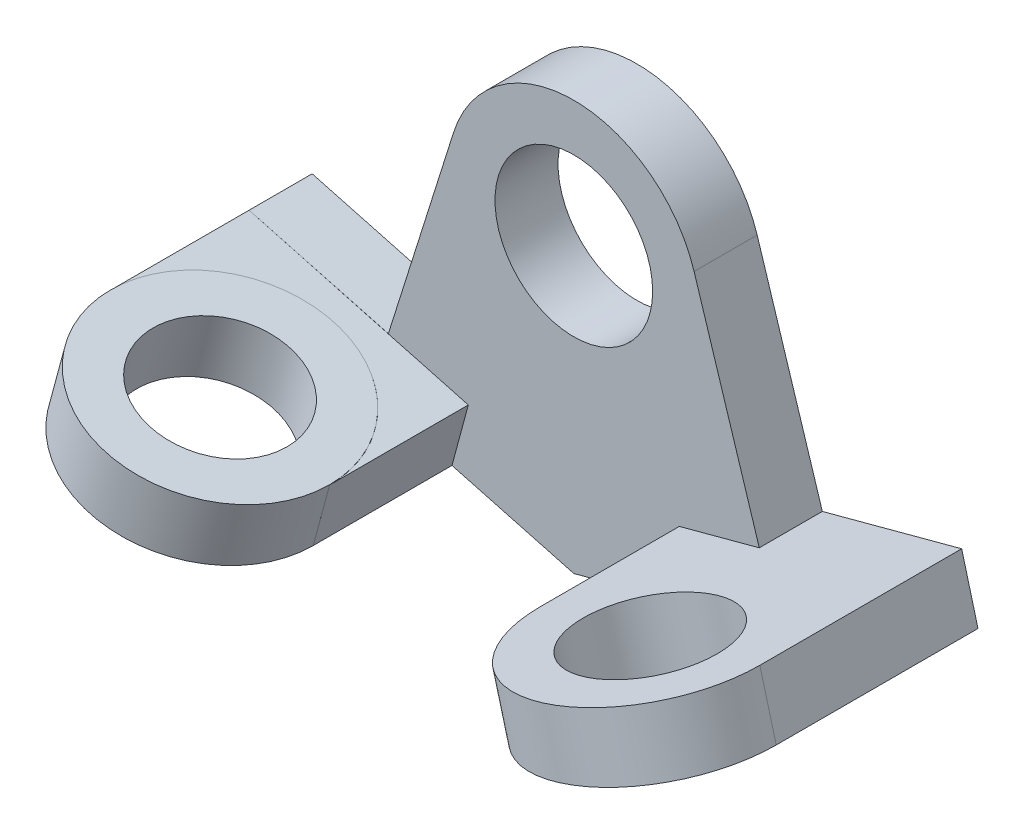
ISO-10303-21;
HEADER;
FILE_DESCRIPTION(('STEP AP214'),'2;1');
FILE_NAME('part.step','',(''),(''),'','','');
FILE_SCHEMA(('AUTOMOTIVE_DESIGN { 1 0 10303 214 1 1 1 1 }'));
ENDSEC;
DATA;
#1=APPLICATION_CONTEXT('core data for automotive mechanical design processes');
#2=APPLICATION_PROTOCOL_DEFINITION('international standard','automotive_design',2000,#1);
#3=PRODUCT_CONTEXT('',#1,'mechanical');
#4=PRODUCT('Part','Part','',(#3));
#5=PRODUCT_RELATED_PRODUCT_CATEGORY('part','',(#4));
#6=PRODUCT_DEFINITION_FORMATION('','',#4);
#7=PRODUCT_DEFINITION_CONTEXT('part definition',#1,'design');
#8=PRODUCT_DEFINITION('design','',#6,#7);
#9=PRODUCT_DEFINITION_SHAPE('','',#8);
#10=(LENGTH_UNIT() NAMED_UNIT(*) SI_UNIT(.MILLI.,.METRE.));
#11=(NAMED_UNIT(*) PLANE_ANGLE_UNIT() SI_UNIT($,.RADIAN.));
#12=(NAMED_UNIT(*) SI_UNIT($,.STERADIAN.) SOLID_ANGLE_UNIT());
#13=UNCERTAINTY_MEASURE_WITH_UNIT(LENGTH_MEASURE(1.E-05),#10,'distance_accuracy_value','');
#14=(GEOMETRIC_REPRESENTATION_CONTEXT(3) GLOBAL_UNCERTAINTY_ASSIGNED_CONTEXT((#13)) GLOBAL_UNIT_ASSIGNED_CONTEXT((#10,
#11,#12)) REPRESENTATION_CONTEXT('',''));
#15=CARTESIAN_POINT('',(0.,0.,0.));
#16=DIRECTION('',(0.,0.,1.));
#17=DIRECTION('',(1.,0.,0.));
#18=AXIS2_PLACEMENT_3D('',#15,#16,#17);
#19=CARTESIAN_POINT('',(0.,0.,10.));
#20=DIRECTION('',(0.,0.,1.));
#21=DIRECTION('',(1.,0.,0.));
#22=AXIS2_PLACEMENT_3D('',#19,#20,#21);
#23=PLANE('',#22);
#24=CARTESIAN_POINT('',(0.,45.,10.));
#25=DIRECTION('',(0.,0.,1.));
#26=DIRECTION('',(1.,0.,0.));
#27=AXIS2_PLACEMENT_3D('',#24,#25,#26);
#28=CIRCLE('',#27,12.5);
#29=CARTESIAN_POINT('',(12.5,45.,10.));
#30=VERTEX_POINT('',#29);
#31=EDGE_CURVE('E424',#30,#30,#28,.T.);
#32=ORIENTED_EDGE('',*,*,#31,.F.);
#33=EDGE_LOOP('',(#32));
#34=FACE_BOUND('',#33,.T.);
#35=DIRECTION('',(0.258819045102522,-0.965925826289068,0.));
#36=VECTOR('',#35,1.);
#37=CARTESIAN_POINT('',(16.7303260747562,14.8356391649411,10.));
#38=LINE('',#37,#36);
#39=CARTESIAN_POINT('',(16.7303260747562,14.8356391649411,10.));
#40=VERTEX_POINT('',#39);
#41=CARTESIAN_POINT('',(19.3185165257814,5.17638090205043,10.));
#42=VERTEX_POINT('',#41);
#43=EDGE_CURVE('E172',#40,#42,#38,.T.);
#44=ORIENTED_EDGE('',*,*,#43,.F.);
#45=DIRECTION('',(-0.965925826289068,-0.258819045102522,0.));
#46=VECTOR('',#45,1.);
#47=CARTESIAN_POINT('',(51.5036558211626,24.1531247886319,10.));
#48=LINE('',#47,#46);
#49=CARTESIAN_POINT('',(29.4101278592332,18.2331818132785,10.));
#50=VERTEX_POINT('',#49);
#51=EDGE_CURVE('E210',#50,#40,#48,.T.);
#52=ORIENTED_EDGE('',*,*,#51,.F.);
#53=DIRECTION('',(0.300705799504267,-0.953716950748229,0.));
#54=VECTOR('',#53,1.);
#55=CARTESIAN_POINT('',(31.9798088328629,10.0831949935828,10.));
#56=LINE('',#55,#54);
#57=CARTESIAN_POINT('',(19.0743390149646,51.0141159900853,10.));
#58=VERTEX_POINT('',#57);
#59=EDGE_CURVE('E284',#58,#50,#56,.T.);
#60=ORIENTED_EDGE('',*,*,#59,.F.);
#61=CARTESIAN_POINT('',(0.,45.,10.));
#62=DIRECTION('',(0.,0.,1.));
#63=DIRECTION('',(1.,0.,0.));
#64=AXIS2_PLACEMENT_3D('',#61,#62,#63);
#65=CIRCLE('',#64,20.);
#66=CARTESIAN_POINT('',(-19.0743390149646,51.0141159900853,10.));
#67=VERTEX_POINT('',#66);
#68=EDGE_CURVE('E337',#58,#67,#65,.T.);
#69=ORIENTED_EDGE('',*,*,#68,.T.);
#70=DIRECTION('',(-0.300705799504267,-0.953716950748229,0.));
#71=VECTOR('',#70,1.);
#72=CARTESIAN_POINT('',(-31.9798088328629,10.0831949935828,10.));
#73=LINE('',#72,#71);
#74=CARTESIAN_POINT('',(-29.4101278592332,18.2331818132785,10.));
#75=VERTEX_POINT('',#74);
#76=EDGE_CURVE('E271',#67,#75,#73,.T.);
#77=ORIENTED_EDGE('',*,*,#76,.T.);
#78=DIRECTION('',(-0.965925826289068,0.258819045102521,0.));
#79=VECTOR('',#78,1.);
#80=CARTESIAN_POINT('',(2.58819045102521,9.65925826289068,10.));
#81=LINE('',#80,#79);
#82=CARTESIAN_POINT('',(-51.4905816094325,24.1496215641571,10.));
#83=VERTEX_POINT('',#82);
#84=EDGE_CURVE('E320',#75,#83,#81,.T.);
#85=ORIENTED_EDGE('',*,*,#84,.T.);
#86=DIRECTION('',(-0.965573757302424,0.260129427802544,0.));
#87=VECTOR('',#86,1.);
#88=CARTESIAN_POINT('',(-51.4905816094325,24.1496215641571,10.));
#89=LINE('',#88,#87);
#90=CARTESIAN_POINT('',(-16.7299263465452,14.7849621632655,10.));
#91=VERTEX_POINT('',#90);
#92=EDGE_CURVE('E357',#91,#83,#89,.T.);
#93=ORIENTED_EDGE('',*,*,#92,.F.);
#94=DIRECTION('',(0.260129427802545,0.965573757302424,0.));
#95=VECTOR('',#94,1.);
#96=CARTESIAN_POINT('',(-16.7299263465452,14.7849621632655,10.));
#97=LINE('',#96,#95);
#98=CARTESIAN_POINT('',(-19.3181864512745,5.17760610474064,10.));
#99=VERTEX_POINT('',#98);
#100=EDGE_CURVE('E365',#99,#91,#97,.T.);
#101=ORIENTED_EDGE('',*,*,#100,.F.);
#102=DIRECTION('',(0.965582925438563,-0.260095394233551,0.));
#103=VECTOR('',#102,1.);
#104=CARTESIAN_POINT('',(-54.079171788662,14.5410403029666,10.));
#105=LINE('',#104,#103);
#106=CARTESIAN_POINT('',(-54.079171788662,14.5410403029666,10.));
#107=VERTEX_POINT('',#106);
#108=EDGE_CURVE('E346',#107,#99,#105,.T.);
#109=ORIENTED_EDGE('',*,*,#108,.F.);
#110=DIRECTION('',(-0.96557375730224,0.260129427803227,0.));
#111=VECTOR('',#110,1.);
#112=CARTESIAN_POINT('',(-0.00705915648429595,-0.0262028648872519,10.));
#113=LINE('',#112,#111);
#114=CARTESIAN_POINT('',(-32.4145115016567,8.70449426866302,10.));
#115=VERTEX_POINT('',#114);
#116=EDGE_CURVE('E312',#115,#107,#113,.T.);
#117=ORIENTED_EDGE('',*,*,#116,.F.);
#118=CARTESIAN_POINT('',(-32.420050633813,8.68692638590632,10.));
#119=VERTEX_POINT('',#118);
#120=EDGE_CURVE('E297',#115,#119,#73,.T.);
#121=ORIENTED_EDGE('',*,*,#120,.T.);
#122=DIRECTION('',(-0.965925826289068,0.258819045102521,0.));
#123=VECTOR('',#122,1.);
#124=CARTESIAN_POINT('',(0.,0.,10.));
#125=LINE('',#124,#123);
#126=CARTESIAN_POINT('',(0.,0.,10.));
#127=VERTEX_POINT('',#126);
#128=EDGE_CURVE('E295',#127,#119,#125,.T.);
#129=ORIENTED_EDGE('',*,*,#128,.F.);
#130=DIRECTION('',(0.965925826289068,0.258819045102521,0.));
#131=VECTOR('',#130,1.);
#132=CARTESIAN_POINT('',(0.,0.,10.));
#133=LINE('',#132,#131);
#134=EDGE_CURVE('E290',#127,#42,#133,.T.);
#135=ORIENTED_EDGE('',*,*,#134,.T.);
#136=EDGE_LOOP('',(#44,#52,#60,#69,#77,#85,#93,#101,#109,#117,#121,#129,#135));
#137=FACE_BOUND('',#136,.T.);
#138=ADVANCED_FACE('F41',(#34,#137),#23,.T.);
#139=CARTESIAN_POINT('',(31.9798088328629,10.0831949935828,10.));
#140=DIRECTION('',(0.953716950748229,0.300705799504267,0.));
#141=DIRECTION('',(-0.300705799504267,0.953716950748229,0.));
#142=AXIS2_PLACEMENT_3D('',#139,#140,#141);
#143=PLANE('',#142);
#144=ORIENTED_EDGE('',*,*,#59,.T.);
#145=DIRECTION('',(0.,0.,-1.));
#146=VECTOR('',#145,1.);
#147=CARTESIAN_POINT('',(29.4101278592332,18.2331818132785,10.));
#148=LINE('',#147,#146);
#149=CARTESIAN_POINT('',(29.4101278592332,18.2331818132785,0.));
#150=VERTEX_POINT('',#149);
#151=EDGE_CURVE('E315',#50,#150,#148,.T.);
#152=ORIENTED_EDGE('',*,*,#151,.T.);
#153=DIRECTION('',(0.300705799504267,-0.953716950748229,0.));
#154=VECTOR('',#153,1.);
#155=CARTESIAN_POINT('',(31.9798088328629,10.0831949935828,0.));
#156=LINE('',#155,#154);
#157=CARTESIAN_POINT('',(19.0743390149646,51.0141159900853,0.));
#158=VERTEX_POINT('',#157);
#159=EDGE_CURVE('E264',#158,#150,#156,.T.);
#160=ORIENTED_EDGE('',*,*,#159,.F.);
#161=DIRECTION('',(0.,0.,-1.));
#162=VECTOR('',#161,1.);
#163=CARTESIAN_POINT('',(19.0743390149646,51.0141159900853,10.));
#164=LINE('',#163,#162);
#165=EDGE_CURVE('E47',#58,#158,#164,.T.);
#166=ORIENTED_EDGE('',*,*,#165,.F.);
#167=EDGE_LOOP('',(#144,#152,#160,#166));
#168=FACE_BOUND('',#167,.T.);
#169=ADVANCED_FACE('F43',(#168),#143,.T.);
#170=CARTESIAN_POINT('',(-31.9798088328629,10.0831949935828,10.));
#171=DIRECTION('',(0.953716950748229,-0.300705799504267,0.));
#172=DIRECTION('',(0.300705799504267,0.953716950748229,0.));
#173=AXIS2_PLACEMENT_3D('',#170,#171,#172);
#174=PLANE('',#173);
#175=DIRECTION('',(0.,0.,1.));
#176=VECTOR('',#175,1.);
#177=CARTESIAN_POINT('',(-32.4145115016567,8.70449426866302,10.));
#178=LINE('',#177,#176);
#179=CARTESIAN_POINT('',(-32.4145115016567,8.70449426866302,0.));
#180=VERTEX_POINT('',#179);
#181=EDGE_CURVE('E299',#180,#115,#178,.T.);
#182=ORIENTED_EDGE('',*,*,#181,.F.);
#183=DIRECTION('',(-0.300705799504267,-0.953716950748229,0.));
#184=VECTOR('',#183,1.);
#185=CARTESIAN_POINT('',(-31.9798088328629,10.0831949935828,0.));
#186=LINE('',#185,#184);
#187=CARTESIAN_POINT('',(-32.420050633813,8.68692638590632,0.));
#188=VERTEX_POINT('',#187);
#189=EDGE_CURVE('E262',#180,#188,#186,.T.);
#190=ORIENTED_EDGE('',*,*,#189,.T.);
#191=DIRECTION('',(0.,0.,-1.));
#192=VECTOR('',#191,1.);
#193=CARTESIAN_POINT('',(-32.420050633813,8.68692638590632,10.));
#194=LINE('',#193,#192);
#195=EDGE_CURVE('E275',#119,#188,#194,.T.);
#196=ORIENTED_EDGE('',*,*,#195,.F.);
#197=ORIENTED_EDGE('',*,*,#120,.F.);
#198=EDGE_LOOP('',(#182,#190,#196,#197));
#199=FACE_BOUND('',#198,.T.);
#200=ADVANCED_FACE('F246',(#199),#174,.F.);
#201=CARTESIAN_POINT('',(0.,45.,10.));
#202=DIRECTION('',(0.,0.,-1.));
#203=DIRECTION('',(-1.,0.,0.));
#204=AXIS2_PLACEMENT_3D('',#201,#202,#203);
#205=CYLINDRICAL_SURFACE('',#204,20.);
#206=CARTESIAN_POINT('',(0.,45.,0.));
#207=DIRECTION('',(0.,0.,1.));
#208=DIRECTION('',(1.,0.,0.));
#209=AXIS2_PLACEMENT_3D('',#206,#207,#208);
#210=CIRCLE('',#209,20.);
#211=CARTESIAN_POINT('',(-19.0743390149646,51.0141159900853,0.));
#212=VERTEX_POINT('',#211);
#213=EDGE_CURVE('E254',#158,#212,#210,.T.);
#214=ORIENTED_EDGE('',*,*,#213,.T.);
#215=DIRECTION('',(0.,0.,-1.));
#216=VECTOR('',#215,1.);
#217=CARTESIAN_POINT('',(-19.0743390149646,51.0141159900853,10.));
#218=LINE('',#217,#216);
#219=EDGE_CURVE('E256',#67,#212,#218,.T.);
#220=ORIENTED_EDGE('',*,*,#219,.F.);
#221=ORIENTED_EDGE('',*,*,#68,.F.);
#222=ORIENTED_EDGE('',*,*,#165,.T.);
#223=EDGE_LOOP('',(#214,#220,#221,#222));
#224=FACE_BOUND('',#223,.T.);
#225=ADVANCED_FACE('F244',(#224),#205,.T.);
#226=CARTESIAN_POINT('',(-29.4101278592332,18.2331818132785,0.));
#227=VERTEX_POINT('',#226);
#228=EDGE_CURVE('E267',#212,#227,#186,.T.);
#229=ORIENTED_EDGE('',*,*,#228,.T.);
#230=DIRECTION('',(0.,0.,1.));
#231=VECTOR('',#230,1.);
#232=CARTESIAN_POINT('',(-29.4101278592332,18.2331818132785,10.));
#233=LINE('',#232,#231);
#234=EDGE_CURVE('E328',#227,#75,#233,.T.);
#235=ORIENTED_EDGE('',*,*,#234,.T.);
#236=ORIENTED_EDGE('',*,*,#76,.F.);
#237=ORIENTED_EDGE('',*,*,#219,.T.);
#238=EDGE_LOOP('',(#229,#235,#236,#237));
#239=FACE_BOUND('',#238,.T.);
#240=ADVANCED_FACE('F242',(#239),#174,.F.);
#241=CARTESIAN_POINT('',(0.,0.,10.));
#242=DIRECTION('',(-0.258819045102521,-0.965925826289068,0.));
#243=DIRECTION('',(0.965925826289068,-0.258819045102521,0.));
#244=AXIS2_PLACEMENT_3D('',#241,#242,#243);
#245=PLANE('',#244);
#246=ORIENTED_EDGE('',*,*,#128,.T.);
#247=ORIENTED_EDGE('',*,*,#195,.T.);
#248=DIRECTION('',(-0.965925826289068,0.258819045102521,0.));
#249=VECTOR('',#248,1.);
#250=CARTESIAN_POINT('',(0.,0.,0.));
#251=LINE('',#250,#249);
#252=CARTESIAN_POINT('',(0.,0.,0.));
#253=VERTEX_POINT('',#252);
#254=EDGE_CURVE('E280',#253,#188,#251,.T.);
#255=ORIENTED_EDGE('',*,*,#254,.F.);
#256=DIRECTION('',(0.,0.,-1.));
#257=VECTOR('',#256,1.);
#258=CARTESIAN_POINT('',(0.,0.,10.));
#259=LINE('',#258,#257);
#260=EDGE_CURVE('E281',#127,#253,#259,.T.);
#261=ORIENTED_EDGE('',*,*,#260,.F.);
#262=EDGE_LOOP('',(#246,#247,#255,#261));
#263=FACE_BOUND('',#262,.T.);
#264=ADVANCED_FACE('F240',(#263),#245,.T.);
#265=CARTESIAN_POINT('',(0.,0.,10.));
#266=DIRECTION('',(-0.258819045102521,0.965925826289068,0.));
#267=DIRECTION('',(-0.965925826289068,-0.258819045102521,0.));
#268=AXIS2_PLACEMENT_3D('',#265,#266,#267);
#269=PLANE('',#268);
#270=CARTESIAN_POINT('',(36.7051813989846,9.83512371389582,32.));
#271=DIRECTION('',(0.258819045102521,-0.965925826289068,0.));
#272=DIRECTION('',(0.965925826289068,0.258819045102521,0.));
#273=AXIS2_PLACEMENT_3D('',#270,#271,#272);
#274=CIRCLE('',#273,11.);
#275=CARTESIAN_POINT('',(47.3303654881643,12.6821332100236,32.));
#276=VERTEX_POINT('',#275);
#277=EDGE_CURVE('E417',#276,#276,#274,.T.);
#278=ORIENTED_EDGE('',*,*,#277,.F.);
#279=EDGE_LOOP('',(#278));
#280=FACE_BOUND('',#279,.T.);
#281=DIRECTION('',(0.,0.,1.));
#282=VECTOR('',#281,1.);
#283=CARTESIAN_POINT('',(54.0918462721878,14.4938665257412,0.));
#284=LINE('',#283,#282);
#285=CARTESIAN_POINT('',(54.0918462721878,14.4938665257412,0.));
#286=VERTEX_POINT('',#285);
#287=CARTESIAN_POINT('',(54.0918462721878,14.4938665257412,32.));
#288=VERTEX_POINT('',#287);
#289=EDGE_CURVE('E165',#286,#288,#284,.T.);
#290=ORIENTED_EDGE('',*,*,#289,.T.);
#291=CARTESIAN_POINT('',(36.7051813989846,9.83512371389582,32.));
#292=DIRECTION('',(0.258819045102521,-0.965925826289068,0.));
#293=DIRECTION('',(0.965925826289068,0.258819045102521,0.));
#294=AXIS2_PLACEMENT_3D('',#291,#292,#293);
#295=CIRCLE('',#294,18.);
#296=CARTESIAN_POINT('',(19.3185165257814,5.17638090205043,32.));
#297=VERTEX_POINT('',#296);
#298=EDGE_CURVE('E180',#288,#297,#295,.T.);
#299=ORIENTED_EDGE('',*,*,#298,.T.);
#300=DIRECTION('',(0.,0.,-1.));
#301=VECTOR('',#300,1.);
#302=CARTESIAN_POINT('',(19.3185165257814,5.17638090205043,32.));
#303=LINE('',#302,#301);
#304=EDGE_CURVE('E349',#297,#42,#303,.T.);
#305=ORIENTED_EDGE('',*,*,#304,.T.);
#306=ORIENTED_EDGE('',*,*,#134,.F.);
#307=ORIENTED_EDGE('',*,*,#260,.T.);
#308=DIRECTION('',(0.965925826289068,0.258819045102521,0.));
#309=VECTOR('',#308,1.);
#310=CARTESIAN_POINT('',(0.,0.,0.));
#311=LINE('',#310,#309);
#312=EDGE_CURVE('E177',#253,#286,#311,.T.);
#313=ORIENTED_EDGE('',*,*,#312,.T.);
#314=EDGE_LOOP('',(#290,#299,#305,#306,#307,#313));
#315=FACE_BOUND('',#314,.T.);
#316=ADVANCED_FACE('F171',(#280,#315),#269,.F.);
#317=CARTESIAN_POINT('',(0.,0.,0.));
#318=DIRECTION('',(0.,0.,1.));
#319=DIRECTION('',(1.,0.,0.));
#320=AXIS2_PLACEMENT_3D('',#317,#318,#319);
#321=PLANE('',#320);
#322=CARTESIAN_POINT('',(0.,45.,0.));
#323=DIRECTION('',(0.,0.,1.));
#324=DIRECTION('',(1.,0.,0.));
#325=AXIS2_PLACEMENT_3D('',#322,#323,#324);
#326=CIRCLE('',#325,12.5);
#327=CARTESIAN_POINT('',(12.5,45.,0.));
#328=VERTEX_POINT('',#327);
#329=EDGE_CURVE('E423',#328,#328,#326,.T.);
#330=ORIENTED_EDGE('',*,*,#329,.T.);
#331=EDGE_LOOP('',(#330));
#332=FACE_BOUND('',#331,.T.);
#333=DIRECTION('',(-0.258819045102521,0.965925826289068,0.));
#334=VECTOR('',#333,1.);
#335=CARTESIAN_POINT('',(54.0918462721878,14.4938665257412,0.));
#336=LINE('',#335,#334);
#337=CARTESIAN_POINT('',(51.5036558211626,24.1531247886319,0.));
#338=VERTEX_POINT('',#337);
#339=EDGE_CURVE('E305',#286,#338,#336,.T.);
#340=ORIENTED_EDGE('',*,*,#339,.F.);
#341=ORIENTED_EDGE('',*,*,#312,.F.);
#342=ORIENTED_EDGE('',*,*,#254,.T.);
#343=ORIENTED_EDGE('',*,*,#189,.F.);
#344=DIRECTION('',(-0.96557375730224,0.260129427803227,0.));
#345=VECTOR('',#344,1.);
#346=CARTESIAN_POINT('',(-0.00705915648429595,-0.0262028648872519,0.));
#347=LINE('',#346,#345);
#348=CARTESIAN_POINT('',(-54.079171788662,14.5410403029666,0.));
#349=VERTEX_POINT('',#348);
#350=EDGE_CURVE('E296',#180,#349,#347,.T.);
#351=ORIENTED_EDGE('',*,*,#350,.T.);
#352=DIRECTION('',(0.260129427803227,0.96557375730224,0.));
#353=VECTOR('',#352,1.);
#354=CARTESIAN_POINT('',(-54.0721126321777,14.5672431678538,0.));
#355=LINE('',#354,#353);
#356=CARTESIAN_POINT('',(-51.4905816094325,24.1496215641571,0.));
#357=VERTEX_POINT('',#356);
#358=EDGE_CURVE('E317',#349,#357,#355,.T.);
#359=ORIENTED_EDGE('',*,*,#358,.T.);
#360=DIRECTION('',(-0.965925826289068,0.258819045102521,0.));
#361=VECTOR('',#360,1.);
#362=CARTESIAN_POINT('',(2.58819045102521,9.65925826289068,0.));
#363=LINE('',#362,#361);
#364=EDGE_CURVE('E277',#227,#357,#363,.T.);
#365=ORIENTED_EDGE('',*,*,#364,.F.);
#366=ORIENTED_EDGE('',*,*,#228,.F.);
#367=ORIENTED_EDGE('',*,*,#213,.F.);
#368=ORIENTED_EDGE('',*,*,#159,.T.);
#369=DIRECTION('',(0.965925826289068,0.258819045102522,0.));
#370=VECTOR('',#369,1.);
#371=CARTESIAN_POINT('',(-2.58819045102522,9.65925826289067,0.));
#372=LINE('',#371,#370);
#373=EDGE_CURVE('E179',#150,#338,#372,.T.);
#374=ORIENTED_EDGE('',*,*,#373,.T.);
#375=EDGE_LOOP('',(#340,#341,#342,#343,#351,#359,#365,#366,#367,#368,#374));
#376=FACE_BOUND('',#375,.T.);
#377=ADVANCED_FACE('F230',(#332,#376),#321,.F.);
#378=CARTESIAN_POINT('',(-0.00705915648429595,-0.0262028648872519,0.));
#379=DIRECTION('',(0.260129427803227,0.96557375730224,0.));
#380=DIRECTION('',(-0.96557375730224,0.260129427803227,0.));
#381=AXIS2_PLACEMENT_3D('',#378,#379,#380);
#382=PLANE('',#381);
#383=ORIENTED_EDGE('',*,*,#350,.F.);
#384=ORIENTED_EDGE('',*,*,#181,.T.);
#385=ORIENTED_EDGE('',*,*,#116,.T.);
#386=DIRECTION('',(0.,0.,1.));
#387=VECTOR('',#386,1.);
#388=CARTESIAN_POINT('',(-54.079171788662,14.5410403029666,0.));
#389=LINE('',#388,#387);
#390=EDGE_CURVE('E326',#349,#107,#389,.T.);
#391=ORIENTED_EDGE('',*,*,#390,.F.);
#392=EDGE_LOOP('',(#383,#384,#385,#391));
#393=FACE_BOUND('',#392,.T.);
#394=ADVANCED_FACE('F224',(#393),#382,.F.);
#395=CARTESIAN_POINT('',(2.58819045102521,9.65925826289068,0.));
#396=DIRECTION('',(0.258819045102521,0.965925826289068,0.));
#397=DIRECTION('',(-0.965925826289068,0.258819045102521,0.));
#398=AXIS2_PLACEMENT_3D('',#395,#396,#397);
#399=PLANE('',#398);
#400=ORIENTED_EDGE('',*,*,#234,.F.);
#401=ORIENTED_EDGE('',*,*,#364,.T.);
#402=DIRECTION('',(0.,0.,1.));
#403=VECTOR('',#402,1.);
#404=CARTESIAN_POINT('',(-51.4905816094325,24.1496215641571,0.));
#405=LINE('',#404,#403);
#406=EDGE_CURVE('E321',#357,#83,#405,.T.);
#407=ORIENTED_EDGE('',*,*,#406,.T.);
#408=ORIENTED_EDGE('',*,*,#84,.F.);
#409=EDGE_LOOP('',(#400,#401,#407,#408));
#410=FACE_BOUND('',#409,.T.);
#411=ADVANCED_FACE('F218',(#410),#399,.T.);
#412=CARTESIAN_POINT('',(-54.0721126321777,14.5672431678538,0.));
#413=DIRECTION('',(0.96557375730224,-0.260129427803227,0.));
#414=DIRECTION('',(0.260129427803227,0.96557375730224,0.));
#415=AXIS2_PLACEMENT_3D('',#412,#413,#414);
#416=PLANE('',#415);
#417=DIRECTION('',(0.,0.,-1.));
#418=VECTOR('',#417,1.);
#419=CARTESIAN_POINT('',(-54.079171788662,14.5410403029666,32.));
#420=LINE('',#419,#418);
#421=CARTESIAN_POINT('',(-54.079171788662,14.5410403029666,32.));
#422=VERTEX_POINT('',#421);
#423=EDGE_CURVE('E302',#422,#107,#420,.T.);
#424=ORIENTED_EDGE('',*,*,#423,.F.);
#425=CARTESIAN_POINT('',(-46.1401790359116,44.0097671832916,31.8032146717555));
#426=CARTESIAN_POINT('',(-47.0312700160347,40.7021288547802,31.8169585458045));
#427=CARTESIAN_POINT('',(-47.9224712652414,37.3940812187401,31.8274072370403));
#428=CARTESIAN_POINT('',(-49.7059957982394,30.7738210693569,31.8520832271609));
#429=CARTESIAN_POINT('',(-50.5983190770658,27.4616085744431,31.8663152833478));
#430=CARTESIAN_POINT('',(-51.880830502518,22.701057696694,31.8969542036948));
#431=CARTESIAN_POINT('',(-52.2711113403579,21.2523752535788,31.9076338418431));
#432=CARTESIAN_POINT('',(-53.0516511470731,18.3550915427025,31.9260451678533));
#433=CARTESIAN_POINT('',(-53.4419099197531,16.9064910031985,31.9337790242718));
#434=CARTESIAN_POINT('',(-53.8803471857861,15.2790568375211,31.9691854977716));
#435=CARTESIAN_POINT('',(-53.9290698320687,15.0982033714825,31.9734920152155));
#436=CARTESIAN_POINT('',(-54.0023212422901,14.8263016493577,31.9799157015397));
#437=CARTESIAN_POINT('',(-54.0267666647991,14.7355627481111,31.982050948051));
#438=CARTESIAN_POINT('',(-54.057079659843,14.6230440193886,31.9898384756815));
#439=CARTESIAN_POINT('',(-54.0631303226298,14.6005845796757,31.9916519986391));
#440=CARTESIAN_POINT('',(-54.0723384643401,14.5664049020283,31.9937483673074));
#441=CARTESIAN_POINT('',(-54.0754316495452,14.5549233157824,31.994343329953));
#442=CARTESIAN_POINT('',(-54.0784235592916,14.5438176536516,31.9980906743327));
#443=CARTESIAN_POINT('',(-54.078513975603,14.5434820375768,31.9982071180463));
#444=CARTESIAN_POINT('',(-54.0786927292111,14.5428185225163,31.9984680987882));
#445=CARTESIAN_POINT('',(-54.0787810531462,14.5424906731278,31.998612779695));
#446=CARTESIAN_POINT('',(-54.0789098030319,14.5420127667564,31.9988642710901));
#447=CARTESIAN_POINT('',(-54.0789523613107,14.5418547947902,31.9989545488307));
#448=CARTESIAN_POINT('',(-54.079032463062,14.5415574653049,31.9991631524438));
#449=CARTESIAN_POINT('',(-54.0790700590702,14.5414179127782,31.9992811401315));
#450=CARTESIAN_POINT('',(-54.0791115045567,14.5412640713829,31.999456813128));
#451=CARTESIAN_POINT('',(-54.079120265523,14.5412315515746,31.9994973112168));
#452=CARTESIAN_POINT('',(-54.0791363654766,14.5411717901979,31.9995824182899));
#453=CARTESIAN_POINT('',(-54.0791437053446,14.5411445453607,31.999627024703));
#454=CARTESIAN_POINT('',(-54.0791548093399,14.541103328469,31.9997098721149));
#455=CARTESIAN_POINT('',(-54.0791590072236,14.5410877463552,31.9997472429509));
#456=CARTESIAN_POINT('',(-54.0791657702645,14.5410626426411,31.9998240796897));
#457=CARTESIAN_POINT('',(-54.0791683400519,14.5410531038535,31.9998635393019));
#458=CARTESIAN_POINT('',(-54.0791714367994,14.5410416090445,31.9999439174113));
#459=CARTESIAN_POINT('',(-54.0791719501165,14.5410397036641,31.99998484384));
#460=CARTESIAN_POINT('',(-54.0791710579264,14.5410430153823,32.0000664986941));
#461=CARTESIAN_POINT('',(-54.0791696442846,14.5410482626758,32.000107225547));
#462=CARTESIAN_POINT('',(-54.0791648423535,14.5410660869515,32.0001907644185));
#463=CARTESIAN_POINT('',(-54.0791612885313,14.5410792783749,32.0002334364471));
#464=CARTESIAN_POINT('',(-54.0791522406452,14.5411128632002,32.0003153205809));
#465=CARTESIAN_POINT('',(-54.0791467582219,14.5411332133931,32.000354551718));
#466=CARTESIAN_POINT('',(-54.0791403690286,14.5411569294236,32.0003914863503));
#467=B_SPLINE_CURVE_WITH_KNOTS('',3,(#425,#426,#427,#428,#429,#430,#431,#432,#433,#434,#435,
#436,#437,#438,#439,#440,#441,#442,#443,#444,#445,#446,#447,#448,#449,#450,#451,#452,#453,#454,
#455,#456,#457,#458,#459,#460,#461,#462,#463,#464,#465,#466),.UNSPECIFIED.,.F.,.F.,(4,2,2,2,2,2,
2,2,2,2,2,2,2,2,2,2,2,2,2,2,4),(0.,10.2776084136231,20.5682017962905,25.0698922193943,
29.5682622591109,30.1307667858114,30.4120277401128,30.482346911265,30.5175461825921,
30.5186454029298,30.5197503777412,30.5203101961429,30.5208635080439,30.5210212776545,
30.5211789491828,30.521300641639,30.5214219864279,30.5215441349135,30.5216668006458,
30.5218004539082,30.5219333139266),.UNSPECIFIED.);
#468=CARTESIAN_POINT('',(-51.4905816094325,24.1496215641571,31.8876311243572));
#469=VERTEX_POINT('',#468);
#470=EDGE_CURVE('E57',#422,#469,#467,.F.);
#471=ORIENTED_EDGE('',*,*,#470,.T.);
#472=DIRECTION('',(0.,0.,-1.));
#473=VECTOR('',#472,1.);
#474=CARTESIAN_POINT('',(-51.4905816094325,24.1496215641571,32.));
#475=LINE('',#474,#473);
#476=EDGE_CURVE('E363',#469,#83,#475,.T.);
#477=ORIENTED_EDGE('',*,*,#476,.T.);
#478=ORIENTED_EDGE('',*,*,#406,.F.);
#479=ORIENTED_EDGE('',*,*,#358,.F.);
#480=ORIENTED_EDGE('',*,*,#390,.T.);
#481=EDGE_LOOP('',(#424,#471,#477,#478,#479,#480));
#482=FACE_BOUND('',#481,.T.);
#483=ADVANCED_FACE('F213',(#482),#416,.F.);
#484=CARTESIAN_POINT('',(-2.58819045102522,9.65925826289067,0.));
#485=DIRECTION('',(0.258819045102522,-0.965925826289068,0.));
#486=DIRECTION('',(0.965925826289068,0.258819045102522,0.));
#487=AXIS2_PLACEMENT_3D('',#484,#485,#486);
#488=PLANE('',#487);
#489=CARTESIAN_POINT('',(34.1169909479594,19.4943819767865,32.));
#490=DIRECTION('',(0.258819045102521,-0.965925826289068,0.));
#491=DIRECTION('',(0.965925826289068,0.258819045102521,0.));
#492=AXIS2_PLACEMENT_3D('',#489,#490,#491);
#493=CIRCLE('',#492,11.);
#494=CARTESIAN_POINT('',(44.7421750371391,22.3413914729142,32.));
#495=VERTEX_POINT('',#494);
#496=EDGE_CURVE('E414',#495,#495,#493,.T.);
#497=ORIENTED_EDGE('',*,*,#496,.T.);
#498=EDGE_LOOP('',(#497));
#499=FACE_BOUND('',#498,.T.);
#500=DIRECTION('',(0.,0.,-1.));
#501=VECTOR('',#500,1.);
#502=CARTESIAN_POINT('',(16.7303260747562,14.8356391649411,32.));
#503=LINE('',#502,#501);
#504=CARTESIAN_POINT('',(16.7303260747562,14.8356391649411,32.));
#505=VERTEX_POINT('',#504);
#506=EDGE_CURVE('E344',#505,#40,#503,.T.);
#507=ORIENTED_EDGE('',*,*,#506,.F.);
#508=CARTESIAN_POINT('',(34.1169909479594,19.4943819767865,32.));
#509=DIRECTION('',(0.258819045102521,-0.965925826289068,0.));
#510=DIRECTION('',(0.965925826289068,0.258819045102521,0.));
#511=AXIS2_PLACEMENT_3D('',#508,#509,#510);
#512=CIRCLE('',#511,18.);
#513=CARTESIAN_POINT('',(51.5036558211626,24.1531247886319,32.));
#514=VERTEX_POINT('',#513);
#515=EDGE_CURVE('E183',#514,#505,#512,.T.);
#516=ORIENTED_EDGE('',*,*,#515,.F.);
#517=DIRECTION('',(0.,0.,1.));
#518=VECTOR('',#517,1.);
#519=CARTESIAN_POINT('',(51.5036558211626,24.1531247886319,0.));
#520=LINE('',#519,#518);
#521=EDGE_CURVE('E164',#338,#514,#520,.T.);
#522=ORIENTED_EDGE('',*,*,#521,.F.);
#523=ORIENTED_EDGE('',*,*,#373,.F.);
#524=ORIENTED_EDGE('',*,*,#151,.F.);
#525=ORIENTED_EDGE('',*,*,#51,.T.);
#526=EDGE_LOOP('',(#507,#516,#522,#523,#524,#525));
#527=FACE_BOUND('',#526,.T.);
#528=ADVANCED_FACE('F217',(#499,#527),#488,.F.);
#529=CARTESIAN_POINT('',(54.0918462721878,14.4938665257412,0.));
#530=DIRECTION('',(0.965925826289068,0.258819045102521,0.));
#531=DIRECTION('',(-0.258819045102521,0.965925826289068,0.));
#532=AXIS2_PLACEMENT_3D('',#529,#530,#531);
#533=PLANE('',#532);
#534=ORIENTED_EDGE('',*,*,#521,.T.);
#535=DIRECTION('',(-0.258819045102521,0.965925826289068,0.));
#536=VECTOR('',#535,1.);
#537=CARTESIAN_POINT('',(54.0918462721878,14.4938665257412,32.));
#538=LINE('',#537,#536);
#539=EDGE_CURVE('E158',#288,#514,#538,.T.);
#540=ORIENTED_EDGE('',*,*,#539,.F.);
#541=ORIENTED_EDGE('',*,*,#289,.F.);
#542=ORIENTED_EDGE('',*,*,#339,.T.);
#543=EDGE_LOOP('',(#534,#540,#541,#542));
#544=FACE_BOUND('',#543,.T.);
#545=ADVANCED_FACE('F159',(#544),#533,.T.);
#546=CARTESIAN_POINT('',(-54.079171788662,14.5410403029666,32.));
#547=DIRECTION('',(0.260095394233551,0.965582925438563,0.));
#548=DIRECTION('',(-0.965582925438563,0.260095394233551,0.));
#549=AXIS2_PLACEMENT_3D('',#546,#547,#548);
#550=PLANE('',#549);
#551=CARTESIAN_POINT('',(-36.6986791199682,9.85932320385362,32.));
#552=DIRECTION('',(-0.260095394233552,-0.965582925438563,0.));
#553=DIRECTION('',(0.965582925438563,-0.260095394233552,0.));
#554=AXIS2_PLACEMENT_3D('',#551,#552,#553);
#555=CIRCLE('',#554,11.);
#556=CARTESIAN_POINT('',(-26.077266940144,6.99827386728455,32.));
#557=VERTEX_POINT('',#556);
#558=EDGE_CURVE('E191',#557,#557,#555,.T.);
#559=ORIENTED_EDGE('',*,*,#558,.F.);
#560=EDGE_LOOP('',(#559));
#561=FACE_BOUND('',#560,.T.);
#562=DIRECTION('',(0.,0.,-1.));
#563=VECTOR('',#562,1.);
#564=CARTESIAN_POINT('',(-19.3181864512745,5.17760610474064,32.));
#565=LINE('',#564,#563);
#566=CARTESIAN_POINT('',(-19.3181864512745,5.17760610474064,32.));
#567=VERTEX_POINT('',#566);
#568=EDGE_CURVE('E306',#567,#99,#565,.T.);
#569=ORIENTED_EDGE('',*,*,#568,.F.);
#570=CARTESIAN_POINT('',(-36.6986791199683,9.85932320385363,32.));
#571=DIRECTION('',(-0.260095394233552,-0.965582925438563,0.));
#572=DIRECTION('',(0.965582925438563,-0.260095394233552,0.));
#573=AXIS2_PLACEMENT_3D('',#570,#571,#572);
#574=CIRCLE('',#573,18.0000000111846);
#575=EDGE_CURVE('E188',#567,#422,#574,.T.);
#576=ORIENTED_EDGE('',*,*,#575,.T.);
#577=ORIENTED_EDGE('',*,*,#423,.T.);
#578=ORIENTED_EDGE('',*,*,#108,.T.);
#579=EDGE_LOOP('',(#569,#576,#577,#578));
#580=FACE_BOUND('',#579,.T.);
#581=ADVANCED_FACE('F378',(#561,#580),#550,.F.);
#582=CARTESIAN_POINT('',(-16.7299263465452,14.7849621632655,32.));
#583=DIRECTION('',(-0.965573757302424,0.260129427802545,0.));
#584=DIRECTION('',(-0.260129427802545,-0.965573757302424,0.));
#585=AXIS2_PLACEMENT_3D('',#582,#583,#584);
#586=PLANE('',#585);
#587=ORIENTED_EDGE('',*,*,#100,.T.);
#588=DIRECTION('',(0.,0.,-1.));
#589=VECTOR('',#588,1.);
#590=CARTESIAN_POINT('',(-16.7299263465452,14.7849621632655,32.));
#591=LINE('',#590,#589);
#592=CARTESIAN_POINT('',(-16.7299263465452,14.7849621632655,32.));
#593=VERTEX_POINT('',#592);
#594=EDGE_CURVE('E367',#593,#91,#591,.T.);
#595=ORIENTED_EDGE('',*,*,#594,.F.);
#596=DIRECTION('',(0.260129427802545,0.965573757302424,0.));
#597=VECTOR('',#596,1.);
#598=CARTESIAN_POINT('',(-16.7299263465452,14.7849621632655,32.));
#599=LINE('',#598,#597);
#600=EDGE_CURVE('E356',#567,#593,#599,.T.);
#601=ORIENTED_EDGE('',*,*,#600,.F.);
#602=ORIENTED_EDGE('',*,*,#568,.T.);
#603=EDGE_LOOP('',(#587,#595,#601,#602));
#604=FACE_BOUND('',#603,.T.);
#605=ADVANCED_FACE('F374',(#604),#586,.F.);
#606=CARTESIAN_POINT('',(-51.4905816094325,24.1496215641571,32.));
#607=DIRECTION('',(-0.260129427802544,-0.965573757302424,0.));
#608=DIRECTION('',(0.965573757302424,-0.260129427802544,0.));
#609=AXIS2_PLACEMENT_3D('',#606,#607,#608);
#610=PLANE('',#609);
#611=ORIENTED_EDGE('',*,*,#476,.F.);
#612=CARTESIAN_POINT('',(-34.1105926283641,19.4673830974754,32.));
#613=DIRECTION('',(-0.260129427802544,-0.965573757302424,0.));
#614=DIRECTION('',(0.965573757302424,-0.260129427802544,0.));
#615=AXIS2_PLACEMENT_3D('',#612,#613,#614);
#616=ELLIPSE('',#615,18.0000000223656,18.0000000111846);
#617=CARTESIAN_POINT('',(-16.7302649753249,14.7850533912116,32.));
#618=VERTEX_POINT('',#617);
#619=EDGE_CURVE('E63',#469,#618,#616,.T.);
#620=ORIENTED_EDGE('',*,*,#619,.T.);
#621=DIRECTION('',(-0.965573757302424,0.260129427802544,0.));
#622=VECTOR('',#621,1.);
#623=CARTESIAN_POINT('',(-51.4905816094325,24.1496215641571,32.));
#624=LINE('',#623,#622);
#625=EDGE_CURVE('E358',#593,#618,#624,.T.);
#626=ORIENTED_EDGE('',*,*,#625,.F.);
#627=ORIENTED_EDGE('',*,*,#594,.T.);
#628=ORIENTED_EDGE('',*,*,#92,.T.);
#629=EDGE_LOOP('',(#611,#620,#626,#627,#628));
#630=FACE_BOUND('',#629,.T.);
#631=ADVANCED_FACE('F397',(#630),#610,.F.);
#632=CARTESIAN_POINT('',(0.,0.,32.));
#633=DIRECTION('',(0.,0.,-1.));
#634=DIRECTION('',(-1.,0.,0.));
#635=AXIS2_PLACEMENT_3D('',#632,#633,#634);
#636=PLANE('',#635);
#637=ORIENTED_EDGE('',*,*,#625,.T.);
#638=DIRECTION('',(-0.260095394233552,-0.965582925438563,0.));
#639=VECTOR('',#638,1.);
#640=CARTESIAN_POINT('',(-16.717232508939,14.8334353591263,32.));
#641=LINE('',#640,#639);
#642=EDGE_CURVE('E11',#618,#567,#641,.T.);
#643=ORIENTED_EDGE('',*,*,#642,.T.);
#644=ORIENTED_EDGE('',*,*,#600,.T.);
#645=EDGE_LOOP('',(#637,#643,#644));
#646=FACE_BOUND('',#645,.T.);
#647=ADVANCED_FACE('F385',(#646),#636,.F.);
#648=CARTESIAN_POINT('',(16.7303260747562,14.8356391649411,32.));
#649=DIRECTION('',(0.965925826289068,0.258819045102522,0.));
#650=DIRECTION('',(-0.258819045102522,0.965925826289068,0.));
#651=AXIS2_PLACEMENT_3D('',#648,#649,#650);
#652=PLANE('',#651);
#653=ORIENTED_EDGE('',*,*,#43,.T.);
#654=ORIENTED_EDGE('',*,*,#304,.F.);
#655=DIRECTION('',(0.258819045102522,-0.965925826289068,0.));
#656=VECTOR('',#655,1.);
#657=CARTESIAN_POINT('',(16.7303260747562,14.8356391649411,32.));
#658=LINE('',#657,#656);
#659=EDGE_CURVE('E168',#505,#297,#658,.T.);
#660=ORIENTED_EDGE('',*,*,#659,.F.);
#661=ORIENTED_EDGE('',*,*,#506,.T.);
#662=EDGE_LOOP('',(#653,#654,#660,#661));
#663=FACE_BOUND('',#662,.T.);
#664=ADVANCED_FACE('F352',(#663),#652,.F.);
#665=CARTESIAN_POINT('',(-34.0977251776327,19.5151524582393,32.));
#666=DIRECTION('',(-0.260095394233552,-0.965582925438563,0.));
#667=DIRECTION('',(0.965582925438563,-0.260095394233552,0.));
#668=AXIS2_PLACEMENT_3D('',#665,#666,#667);
#669=CYLINDRICAL_SURFACE('',#668,18.0000000111846);
#670=CARTESIAN_POINT('',(-34.0977251776327,19.5151524582393,32.));
#671=DIRECTION('',(-0.260095394233552,-0.965582925438563,0.));
#672=DIRECTION('',(0.965582925438563,-0.260095394233552,0.));
#673=AXIS2_PLACEMENT_3D('',#670,#671,#672);
#674=CIRCLE('',#673,18.0000000111846);
#675=CARTESIAN_POINT('',(-16.717232508939,14.8334353591263,32.));
#676=VERTEX_POINT('',#675);
#677=EDGE_CURVE('E194',#676,#676,#674,.T.);
#678=ORIENTED_EDGE('',*,*,#677,.T.);
#679=EDGE_LOOP('',(#678));
#680=FACE_BOUND('',#679,.T.);
#681=ORIENTED_EDGE('',*,*,#470,.F.);
#682=ORIENTED_EDGE('',*,*,#575,.F.);
#683=ORIENTED_EDGE('',*,*,#642,.F.);
#684=ORIENTED_EDGE('',*,*,#619,.F.);
#685=EDGE_LOOP('',(#681,#682,#683,#684));
#686=FACE_BOUND('',#685,.T.);
#687=ADVANCED_FACE('F207',(#680,#686),#669,.T.);
#688=CARTESIAN_POINT('',(-34.0977251776327,19.5151524582393,32.));
#689=DIRECTION('',(-0.260095394233552,-0.965582925438563,0.));
#690=DIRECTION('',(0.965582925438563,-0.260095394233552,0.));
#691=AXIS2_PLACEMENT_3D('',#688,#689,#690);
#692=PLANE('',#691);
#693=CARTESIAN_POINT('',(-34.0977251776327,19.5151524582393,32.));
#694=DIRECTION('',(-0.260095394233552,-0.965582925438563,0.));
#695=DIRECTION('',(0.965582925438563,-0.260095394233552,0.));
#696=AXIS2_PLACEMENT_3D('',#693,#694,#695);
#697=CIRCLE('',#696,11.);
#698=CARTESIAN_POINT('',(-23.4763129978085,16.6541031216702,32.));
#699=VERTEX_POINT('',#698);
#700=EDGE_CURVE('E187',#699,#699,#697,.T.);
#701=ORIENTED_EDGE('',*,*,#700,.T.);
#702=EDGE_LOOP('',(#701));
#703=FACE_BOUND('',#702,.T.);
#704=ORIENTED_EDGE('',*,*,#677,.F.);
#705=EDGE_LOOP('',(#704));
#706=FACE_BOUND('',#705,.T.);
#707=ADVANCED_FACE('F384',(#703,#706),#692,.F.);
#708=CARTESIAN_POINT('',(34.1169909479594,19.4943819767865,32.));
#709=DIRECTION('',(0.258819045102521,-0.965925826289068,0.));
#710=DIRECTION('',(0.965925826289068,0.258819045102521,0.));
#711=AXIS2_PLACEMENT_3D('',#708,#709,#710);
#712=CYLINDRICAL_SURFACE('',#711,18.);
#713=ORIENTED_EDGE('',*,*,#515,.T.);
#714=ORIENTED_EDGE('',*,*,#659,.T.);
#715=ORIENTED_EDGE('',*,*,#298,.F.);
#716=ORIENTED_EDGE('',*,*,#539,.T.);
#717=EDGE_LOOP('',(#713,#714,#715,#716));
#718=FACE_BOUND('',#717,.T.);
#719=ADVANCED_FACE('F181',(#718),#712,.T.);
#720=CARTESIAN_POINT('',(-34.0977251776327,19.5151524582393,32.));
#721=DIRECTION('',(-0.260095394233552,-0.965582925438563,0.));
#722=DIRECTION('',(0.965582925438563,-0.260095394233552,0.));
#723=AXIS2_PLACEMENT_3D('',#720,#721,#722);
#724=CYLINDRICAL_SURFACE('',#723,11.);
#725=ORIENTED_EDGE('',*,*,#700,.F.);
#726=EDGE_LOOP('',(#725));
#727=FACE_BOUND('',#726,.T.);
#728=ORIENTED_EDGE('',*,*,#558,.T.);
#729=EDGE_LOOP('',(#728));
#730=FACE_BOUND('',#729,.T.);
#731=ADVANCED_FACE('F524',(#727,#730),#724,.F.);
#732=CARTESIAN_POINT('',(34.1169909479594,19.4943819767865,32.));
#733=DIRECTION('',(0.258819045102521,-0.965925826289068,0.));
#734=DIRECTION('',(0.965925826289068,0.258819045102521,0.));
#735=AXIS2_PLACEMENT_3D('',#732,#733,#734);
#736=CYLINDRICAL_SURFACE('',#735,11.);
#737=ORIENTED_EDGE('',*,*,#496,.F.);
#738=EDGE_LOOP('',(#737));
#739=FACE_BOUND('',#738,.T.);
#740=ORIENTED_EDGE('',*,*,#277,.T.);
#741=EDGE_LOOP('',(#740));
#742=FACE_BOUND('',#741,.T.);
#743=ADVANCED_FACE('F433',(#739,#742),#736,.F.);
#744=CARTESIAN_POINT('',(0.,45.,0.));
#745=DIRECTION('',(0.,0.,1.));
#746=DIRECTION('',(1.,0.,0.));
#747=AXIS2_PLACEMENT_3D('',#744,#745,#746);
#748=CYLINDRICAL_SURFACE('',#747,12.5);
#749=ORIENTED_EDGE('',*,*,#329,.F.);
#750=EDGE_LOOP('',(#749));
#751=FACE_BOUND('',#750,.T.);
#752=ORIENTED_EDGE('',*,*,#31,.T.);
#753=EDGE_LOOP('',(#752));
#754=FACE_BOUND('',#753,.T.);
#755=ADVANCED_FACE('F429',(#751,#754),#748,.F.);
#756=CLOSED_SHELL('',(#138,#169,#200,#225,#240,#264,#316,#377,#394,#411,#483,#528,#545,#581,
#605,#631,#647,#664,#687,#707,#719,#731,#743,#755));
#757=MANIFOLD_SOLID_BREP('B2',#756);
#758=ADVANCED_BREP_SHAPE_REPRESENTATION('',(#18,#757),#14);
#759=SHAPE_DEFINITION_REPRESENTATION(#9,#758);
ENDSEC;
END-ISO-10303-21;
